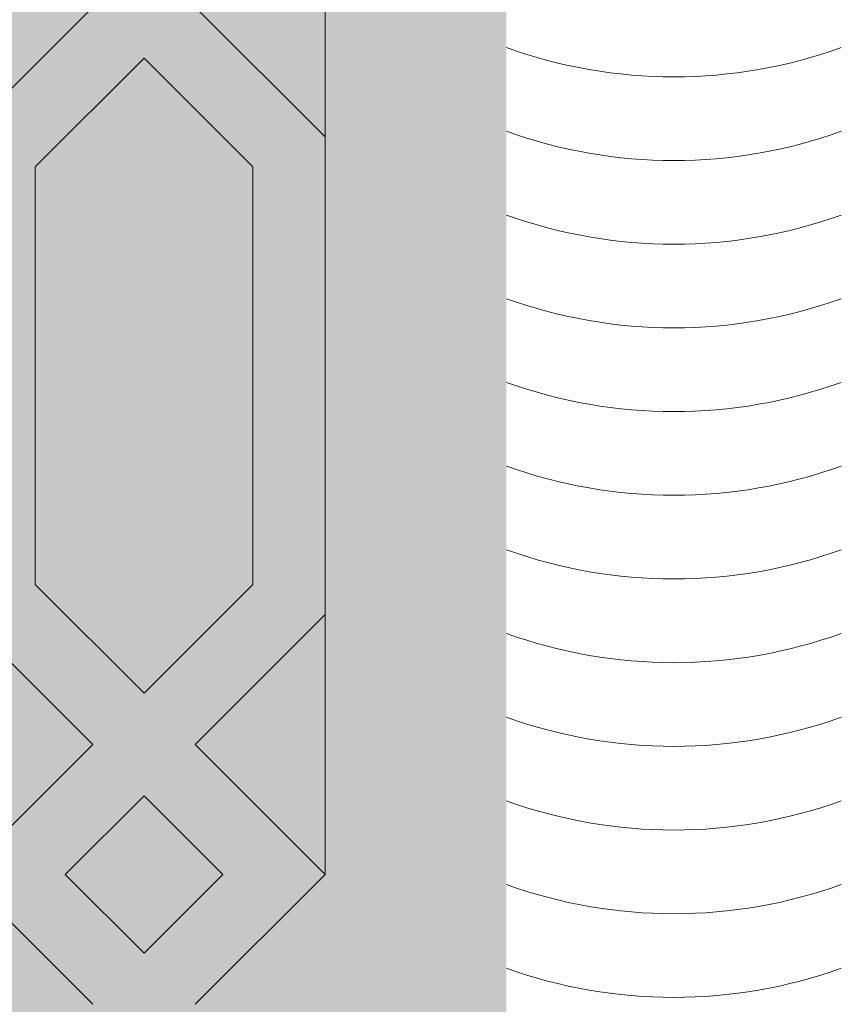
# Model space of a CAD drawing. Units: inches. Extents: x 844 to 2234, y 346 to 1084.
# Tile 37 of 93: x 1262.676 to 1265.567, y 695.763 to 699.229. Entities that reach past the tile are written whole.
import ezdxf

# ---------------------------------------------------------------- set-up
doc = ezdxf.new("R2010")
doc.units = ezdxf.units.IN
doc.header["$MEASUREMENT"] = 0
doc.layers.add('furniture', color=8, linetype='Continuous', lineweight=18)
doc.layers.add('RA-AP-01$0$INT', color=35, linetype='Continuous', lineweight=5)
doc.layers.add('RA-AP-01$0$FURN', color=3, linetype='Continuous')

# ---------------------------------------------------------------- blocks, each defined once
blk = doc.blocks.new('A$C18D01794')
at = {"layer": 'RA-AP-01$0$INT'}
h = blk.add_hatch(color=256, dxfattribs=at)
h.paths.add_polyline_path([(4.355206456958071, -6.156712009588037), (4.355206456958071, -8.056712009588038), (5.455206456958072, -8.056712009588038), (5.455206456958072, -6.156712009588037)])
h.paths.add_polyline_path([(4.405206456958072, -8.006712009588039), (4.405206456958072, -6.206712009588038), (5.405206456958072, -6.206712009588038), (5.405206456958072, -8.006712009588039)], flags=16)
h = blk.add_hatch(color=256, dxfattribs=at)
h.paths.add_polyline_path([(4.469348592586677, -7.07085414521094), (4.505206456958073, -7.03499628085108), (4.505206456958071, -7.106712009593861)])
h.paths.add_polyline_path([(4.455206456960671, -7.084996280832395), (4.476922185709333, -7.106712009588038), (4.433490728198045, -7.106712009588038)])
h.paths.add_polyline_path([(4.405206456958073, -7.034996280813718), (4.441064321339218, -7.070854145206393), (4.40520645695807, -7.106712009576003)])
h.paths.add_polyline_path([(4.425206456989053, -6.911460746921742), (4.455206456990736, -6.881460746929706), (4.485206456989055, -6.911460746937677), (4.48520645696979, -7.026712009590022), (4.455206456965227, -7.056712009584936), (4.425206456969784, -7.026712009579853)])
h.paths.add_polyline_path([(4.505206456958073, -6.831460746955388), (4.505206456958071, -6.903176475661116), (4.469348592616738, -6.867318611308251)])
h.paths.add_polyline_path([(4.425206456964688, -6.707925213036777), (4.455206456964794, -6.677925213027025), (4.485206456964689, -6.707925213017265), (4.485206456983951, -6.823176475683938), (4.455206456990736, -6.853176475686799), (4.425206456983956, -6.823176475689667)])
h.paths.add_polyline_path([(4.425206456974126, -6.504389679118949), (4.455206456959092, -6.474389679124341), (4.485206456974132, -6.504389679129721), (4.485206456993396, -6.619640941768059), (4.45520645699153, -6.649640941779566), (4.425206456993394, -6.619640941791077)])
h.paths.add_polyline_path([(4.46934859260189, -6.663783077416661), (4.505206456958071, -6.627925213048953), (4.505206456958073, -6.699640941761311)])
h.paths.add_polyline_path([(4.405206456958073, -6.627925213005104), (4.441064321354427, -6.663783077389926), (4.405206456958072, -6.699640941797813)])
h.paths.add_polyline_path([(4.405206456958072, -6.424389679139403), (4.441064321333084, -6.460247543502882), (4.405206456958072, -6.496105407889427)])
h.paths.add_polyline_path([(4.469348592580547, -6.460247543498336), (4.505206456958071, -6.424389679109282), (4.505206456958071, -6.496105407864332)])
h.paths.add_polyline_path([(4.425206456957888, -6.300854145208262), (4.45520645695415, -6.270854145221655), (4.485206456959507, -6.300854145217359), (4.48520645695824, -6.416105407863534), (4.455206456954537, -6.44610540787688), (4.425206456957888, -6.416105407889874)])
h.paths.add_polyline_path([(4.425206456957888, -6.226712009591025), (4.471064321332215, -6.226712009591025), (4.425206456957888, -6.272569873980103)])
h.paths.add_polyline_path([(4.499348592575121, -6.226712009591029), (4.636064321343707, -6.226712009591025), (4.666064321342317, -6.256712009589254), (4.636064321340932, -6.286712009591028), (4.499348592588945, -6.286712009591028), (4.469348592591685, -6.256712009584116)])
h.paths.add_polyline_path([(4.680206456964641, -6.270854145214393), (4.716064321337824, -6.306712009588038), (4.644348592591454, -6.306712009588038)])
h.paths.add_polyline_path([(4.644348592588108, -6.206712009588038), (4.716064321341167, -6.206712009588038), (4.680206456964637, -6.242569873964111)])
h.paths.add_polyline_path([(4.724348592586768, -6.226712009589824), (4.861064321340514, -6.226712009589824), (4.891064321340324, -6.256712009589255), (4.861064321340141, -6.286712009589827), (4.724348592587134, -6.286712009589821), (4.694348592586957, -6.256712009589254)])
h.paths.add_polyline_path([(4.905206456964143, -6.270854145212892), (4.941064321338827, -6.306712009588038), (4.869348592589457, -6.306712009588039)])
h.paths.add_polyline_path([(4.869348592586113, -6.206712009588038), (4.941064321342172, -6.206712009588038), (4.905206456964145, -6.242569873965612)])
h.paths.add_polyline_path([(4.949348592587774, -6.226712009589824), (5.086064321341521, -6.226712009589824), (5.116064321341329, -6.256712009589252), (5.08606432134115, -6.286712009589823), (4.949348592588145, -6.286712009589827), (4.919348592587961, -6.256712009589255)])
h.paths.add_polyline_path([(5.130206456963645, -6.270854145214393), (5.166064321336834, -6.306712009588038), (5.094348592590464, -6.306712009588038)])
h.paths.add_polyline_path([(5.094348592587119, -6.206712009588038), (5.166064321340178, -6.206712009588038), (5.130206456963651, -6.242569873964107)])
h.paths.add_polyline_path([(5.174348592584578, -6.226712009591027), (5.311064321353163, -6.226712009591027), (5.341064321336602, -6.256712009584116), (5.31106432133934, -6.286712009591028), (5.174348592587352, -6.286712009591028), (5.144348592585969, -6.256712009589254)])
h.paths.add_polyline_path([(5.325206456968778, -6.300854145217359), (5.355206456974136, -6.270854145221653), (5.385206456970396, -6.300854145208262), (5.385206456970396, -6.416105407889878), (5.355206456973747, -6.44610540787688), (5.325206456970044, -6.416105407863533)])
h.paths.add_polyline_path([(5.339348592596073, -6.226712009591029), (5.385206456970396, -6.226712009591025), (5.385206456970398, -6.272569873980105)])
h.paths.add_polyline_path([(5.325206456954155, -6.504389679129722), (5.355206456969194, -6.474389679124342), (5.38520645695416, -6.504389679118949), (5.385206456934896, -6.619640941791077), (5.355206456936758, -6.649640941779564), (5.325206456934888, -6.619640941768057)])
h.paths.add_polyline_path([(5.305206456958072, -6.424389679097139), (5.341064321347739, -6.460247543498338), (5.305206456958072, -6.496105407876472)])
h.paths.add_polyline_path([(5.369348592595204, -6.460247543502882), (5.40520645695807, -6.42438967915155), (5.405206456958072, -6.496105407877278)])
h.paths.add_polyline_path([(5.405206456958072, -6.627925213017245), (5.405206456958072, -6.69964094178567), (5.369348592573857, -6.663783077389926)])
h.paths.add_polyline_path([(5.305206456958072, -6.62792521303681), (5.341064321326393, -6.663783077416663), (5.305206456958072, -6.69964094177345)])
h.paths.add_polyline_path([(5.325206456963599, -6.707925213017267), (5.355206456963494, -6.677925213027021), (5.385206456963598, -6.707925213036775), (5.385206456944334, -6.823176475689665), (5.355206456937552, -6.853176475686797), (5.325206456944333, -6.823176475683936)])
h.paths.add_polyline_path([(5.305206456958072, -6.831460746943246), (5.341064321311551, -6.867318611308252), (5.305206456958072, -6.903176475673257)])
h.paths.add_polyline_path([(5.325206456939231, -6.911460746937672), (5.355206456937552, -6.881460746929707), (5.385206456939235, -6.911460746921742), (5.385206456958502, -7.026712009579853), (5.355206456963061, -7.056712009584934), (5.3252064569585, -7.026712009590026)])
h.paths.add_polyline_path([(5.404581768715993, -6.832085435167151, 0.001217816984214), (5.405206456958072, -6.832312009593747), (5.405206456958072, -6.90317647569123), (5.369348592563558, -6.867318611308251)])
h.paths.add_polyline_path([(5.36934859258907, -7.070854145206393), (5.40520645695807, -7.034996280825861), (5.405206456958072, -7.106712009563858)])
h.paths.add_polyline_path([(5.355206456967613, -7.084996280832394), (5.376922185730239, -7.106712009588038), (5.333490728218953, -7.106712009588036)])
h.paths.add_polyline_path([(5.30520645695807, -7.034996280838937), (5.341064321341609, -7.070854145210942), (5.305206456958074, -7.106712009606006)])
h = blk.add_hatch(color=256, dxfattribs=at)
h.paths.add_polyline_path([(4.505206456958071, -6.627925213048953), (4.46934859260189, -6.663783077416663), (4.505206456958071, -6.699640941761309), (4.505206456958071, -6.831460746955389), (4.469348592616735, -6.867318611308252), (4.505206456958071, -6.903176475661112), (4.505206456958071, -7.03499628085108), (4.469348592586679, -7.070854145210939), (4.505206456952245, -7.106712009588038), (4.476922185709333, -7.106712009588038), (4.455206456960671, -7.084996280832395), (4.433490728198047, -7.106712009588038), (4.405206456946033, -7.10671200958804), (4.441064321339216, -7.070854145206393), (4.40520645695807, -7.034996280813718), (4.405206456958072, -6.903176475703379), (4.441064321364728, -6.867318611308251), (4.40520645695807, -6.83146074691313), (4.40520645695807, -6.699640941797813), (4.441064321354429, -6.663783077389924), (4.405206456958072, -6.627925213005102), (4.405206456958072, -6.496105407889425), (4.441064321333084, -6.460247543502882), (4.405206456958072, -6.424389679139403), (4.405206456958072, -6.206712009588038), (4.644348592588106, -6.206712009588038), (4.680206456964639, -6.242569873964107), (4.716064321341165, -6.206712009588038), (4.869348592586113, -6.206712009588038), (4.905206456964143, -6.24256987396561), (4.941064321342174, -6.206712009588038), (5.094348592587118, -6.206712009588038), (5.130206456963649, -6.242569873964107), (5.166064321340178, -6.206712009588038), (5.405206456958072, -6.206712009588038), (5.405206456958072, -6.42438967915155), (5.369348592595202, -6.46024754350288), (5.40520645695807, -6.49610540787728), (5.40520645695807, -6.627925213017247), (5.369348592573859, -6.663783077389926), (5.40520645695807, -6.699640941785666), (5.40520645695807, -6.831460746925273), (5.36934859256356, -6.867318611308252), (5.405206456958072, -6.90317647569123), (5.405206456958072, -7.034996280825859), (5.369348592589068, -7.070854145206395), (5.405206456982249, -7.106712009588038), (5.376922185730244, -7.106712009588038), (5.355206456967613, -7.084996280832397), (5.333490728218955, -7.106712009588036), (5.305206456976043, -7.106712009588035), (5.341064321341609, -7.07085414521094), (5.305206456958072, -7.034996280838935), (5.305206456958072, -6.90317647567326), (5.34106432131155, -6.867318611308252), (5.305206456958072, -6.831460746943244), (5.30520645695807, -6.699640941773452), (5.341064321326395, -6.663783077416663), (5.305206456958072, -6.627925213036814), (5.305206456958072, -6.496105407876472), (5.341064321347738, -6.46024754349834), (5.305206456958072, -6.424389679097137), (5.30520645695807, -6.306712009588038), (5.166064321336834, -6.306712009588038), (5.130206456963647, -6.270854145214393), (5.094348592590464, -6.306712009588038), (4.941064321338827, -6.306712009588036), (4.905206456964145, -6.270854145212892), (4.869348592589459, -6.306712009588038), (4.716064321337822, -6.306712009588036), (4.680206456964641, -6.270854145214393), (4.644348592591453, -6.306712009588038), (4.505206456958071, -6.306712009588038), (4.505206456958071, -6.424389679109282), (4.469348592580545, -6.460247543498338), (4.505206456958071, -6.496105407864328)])
h.paths.add_polyline_path([(4.485206456974132, -6.504389679129722), (4.45520645695909, -6.474389679124341), (4.425206456974128, -6.504389679118945), (4.425206456993394, -6.619640941791079), (4.45520645699153, -6.649640941779566), (4.485206456993396, -6.619640941768059)], flags=16)
h.paths.add_polyline_path([(4.455206456954537, -6.44610540787688), (4.485206456958242, -6.416105407863534), (4.48520645695951, -6.30085414521736), (4.45520645695415, -6.270854145221653), (4.425206456957888, -6.300854145208264), (4.425206456957888, -6.41610540788988)], flags=16)
h.paths.add_polyline_path([(4.455206456964794, -6.677925213027025), (4.42520645696469, -6.707925213036777), (4.425206456983954, -6.82317647568967), (4.455206456990734, -6.853176475686797), (4.485206456983953, -6.823176475683936), (4.485206456964687, -6.707925213017265)], flags=16)
h.paths.add_polyline_path([(4.499348592588947, -6.286712009591028), (4.636064321340932, -6.286712009591028), (4.666064321342317, -6.256712009589254), (4.636064321343707, -6.226712009591027), (4.499348592575121, -6.226712009591029), (4.469348592591685, -6.256712009584118)], flags=16)
h.paths.add_polyline_path([(4.425206456957888, -6.272569873980103), (4.471064321332215, -6.226712009591025), (4.425206456957888, -6.226712009591025)], flags=16)
h.paths.add_polyline_path([(4.455206456990734, -6.881460746929709), (4.425206456989053, -6.91146074692174), (4.425206456969784, -7.026712009579853), (4.455206456965226, -7.056712009584932), (4.485206456969787, -7.026712009590026), (4.485206456989053, -6.911460746937672)], flags=16)
h.paths.add_polyline_path([(4.72434859258714, -6.286712009589821), (4.861064321340141, -6.286712009589829), (4.891064321340324, -6.256712009589254), (4.861064321340513, -6.226712009589823), (4.724348592586768, -6.226712009589823), (4.694348592586956, -6.256712009589254)], flags=16)
h.paths.add_polyline_path([(4.919348592587961, -6.256712009589254), (4.949348592588145, -6.286712009589827), (5.08606432134115, -6.286712009589823), (5.116064321341327, -6.256712009589254), (5.086064321341519, -6.226712009589824), (4.949348592587774, -6.226712009589824)], flags=16)
h.paths.add_polyline_path([(5.144348592585967, -6.256712009589254), (5.174348592587358, -6.286712009591028), (5.311064321339338, -6.286712009591028), (5.3410643213366, -6.256712009584118), (5.311064321353163, -6.226712009591029), (5.174348592584576, -6.226712009591027)], flags=16)
h.paths.add_polyline_path([(5.32520645693489, -6.619640941768055), (5.355206456936755, -6.649640941779566), (5.385206456934894, -6.619640941791079), (5.38520645695416, -6.504389679118949), (5.355206456969194, -6.474389679124341), (5.325206456954153, -6.504389679129724)], flags=16)
h.paths.add_polyline_path([(5.325206456970042, -6.416105407863534), (5.355206456973747, -6.44610540787688), (5.385206456970398, -6.416105407889876), (5.385206456970398, -6.30085414520826), (5.355206456974136, -6.270854145221653), (5.325206456968778, -6.30085414521736)], flags=16)
h.paths.add_polyline_path([(5.325206456963599, -6.707925213017265), (5.325206456944333, -6.823176475683936), (5.355206456937552, -6.853176475686797), (5.385206456944332, -6.823176475689667), (5.385206456963596, -6.707925213036773), (5.355206456963492, -6.677925213027027)], flags=16)
h.paths.add_polyline_path([(5.32520645693923, -6.911460746937674), (5.3252064569585, -7.026712009590026), (5.355206456963062, -7.056712009584934), (5.3852064569585, -7.026712009579853), (5.385206456939234, -6.911460746921738), (5.355206456937552, -6.881460746929707)], flags=16)
h.paths.add_polyline_path([(5.339348592596071, -6.226712009591029), (5.385206456970398, -6.272569873980103), (5.385206456970396, -6.226712009591027)], flags=16)
h = blk.add_hatch(color=256, dxfattribs=at)
h.paths.add_polyline_path([(4.505206456958071, -7.585498806127123), (4.46934859260189, -7.549640941759413), (4.505206456958071, -7.513783077414768), (4.505206456958071, -7.381963272220687), (4.469348592616735, -7.346105407867824), (4.505206456958071, -7.310247543514964), (4.505206456958071, -7.178427738324996), (4.469348592586679, -7.142569873965138), (4.505206456952245, -7.106712009588038), (4.476922185709333, -7.106712009588038), (4.455206456960671, -7.128427738343681), (4.433490728198047, -7.106712009588038), (4.405206456946033, -7.106712009588036), (4.441064321339216, -7.142569873969684), (4.40520645695807, -7.178427738362358), (4.405206456958072, -7.310247543472698), (4.441064321364728, -7.346105407867826), (4.40520645695807, -7.381963272262947), (4.40520645695807, -7.513783077378263), (4.441064321354429, -7.549640941786153), (4.405206456958072, -7.585498806170974), (4.405206456958072, -7.717318611286652), (4.441064321333084, -7.753176475673194), (4.405206456958072, -7.789034340036673), (4.405206456958072, -8.006712009588039), (4.644348592588106, -8.006712009588039), (4.680206456964639, -7.970854145211967), (4.716064321341165, -8.006712009588039), (4.869348592586113, -8.006712009588039), (4.905206456964143, -7.970854145210465), (4.941064321342174, -8.006712009588039), (5.094348592587118, -8.006712009588037), (5.130206456963649, -7.970854145211967), (5.166064321340178, -8.006712009588039), (5.405206456958072, -8.006712009588039), (5.405206456958072, -7.789034340024526), (5.369348592595202, -7.753176475673196), (5.40520645695807, -7.717318611298797), (5.40520645695807, -7.585498806158829), (5.369348592573859, -7.549640941786151), (5.40520645695807, -7.51378307739041), (5.40520645695807, -7.381963272250803), (5.36934859256356, -7.346105407867824), (5.405206456958072, -7.310247543484846), (5.405206456958072, -7.178427738350217), (5.369348592589068, -7.142569873969682), (5.405206456982249, -7.106712009588038), (5.376922185730244, -7.106712009588038), (5.355206456967613, -7.128427738343679), (5.333490728218955, -7.10671200958804), (5.305206456976043, -7.106712009588042), (5.341064321341609, -7.142569873965136), (5.305206456958072, -7.178427738337141), (5.305206456958072, -7.310247543502816), (5.34106432131155, -7.346105407867824), (5.305206456958072, -7.381963272232832), (5.30520645695807, -7.513783077402624), (5.341064321326395, -7.549640941759413), (5.305206456958072, -7.585498806139263), (5.305206456958072, -7.717318611299605), (5.341064321347738, -7.753176475677737), (5.305206456958072, -7.78903434007894), (5.30520645695807, -7.906712009588039), (5.166064321336834, -7.906712009588039), (5.130206456963647, -7.942569873961684), (5.094348592590464, -7.906712009588039), (4.941064321338827, -7.906712009588041), (4.905206456964145, -7.942569873963183), (4.869348592589459, -7.906712009588039), (4.716064321337822, -7.906712009588041), (4.680206456964641, -7.942569873961684), (4.644348592591453, -7.906712009588039), (4.505206456958071, -7.906712009588039), (4.505206456958071, -7.789034340066795), (4.469348592580545, -7.753176475677738), (4.505206456958071, -7.717318611311748)])
h.paths.add_polyline_path([(4.485206456974132, -7.709034340046354), (4.45520645695909, -7.739034340051736), (4.425206456974128, -7.709034340057131), (4.425206456993394, -7.593783077384998), (4.45520645699153, -7.563783077396511), (4.485206456993396, -7.593783077408017)], flags=16)
h.paths.add_polyline_path([(4.455206456954537, -7.767318611299197), (4.485206456958242, -7.797318611312542), (4.48520645695951, -7.912569873958716), (4.45520645695415, -7.942569873954422), (4.425206456957888, -7.912569873967813), (4.425206456957888, -7.797318611286197)], flags=16)
h.paths.add_polyline_path([(4.455206456964794, -7.535498806149051), (4.42520645696469, -7.5054988061393), (4.425206456983954, -7.390247543486406), (4.455206456990734, -7.360247543489279), (4.485206456983953, -7.39024754349214), (4.485206456964687, -7.505498806158811)], flags=16)
h.paths.add_polyline_path([(4.499348592588947, -7.926712009585049), (4.636064321340932, -7.926712009585049), (4.666064321342317, -7.956712009586821), (4.636064321343707, -7.986712009585048), (4.499348592575121, -7.986712009585048), (4.469348592591685, -7.956712009591957)], flags=16)
h.paths.add_polyline_path([(4.425206456957888, -7.940854145195974), (4.471064321332215, -7.986712009585049), (4.425206456957888, -7.986712009585049)], flags=16)
h.paths.add_polyline_path([(4.455206456990734, -7.331963272246367), (4.425206456989053, -7.301963272254337), (4.425206456969784, -7.186712009596224), (4.455206456965226, -7.156712009591144), (4.485206456969787, -7.186712009586051), (4.485206456989053, -7.301963272238404)], flags=16)
h.paths.add_polyline_path([(4.72434859258714, -7.926712009586255), (4.861064321340141, -7.926712009586248), (4.891064321340324, -7.956712009586823), (4.861064321340513, -7.986712009586252), (4.724348592586768, -7.986712009586252), (4.694348592586956, -7.956712009586821)], flags=16)
h.paths.add_polyline_path([(4.919348592587961, -7.956712009586821), (4.949348592588145, -7.92671200958625), (5.08606432134115, -7.926712009586253), (5.116064321341327, -7.956712009586823), (5.086064321341519, -7.986712009586252), (4.949348592587774, -7.986712009586252)], flags=16)
h.paths.add_polyline_path([(5.144348592585967, -7.956712009586823), (5.174348592587358, -7.926712009585049), (5.311064321339338, -7.926712009585049), (5.3410643213366, -7.956712009591957), (5.311064321353163, -7.986712009585048), (5.174348592584576, -7.986712009585048)], flags=16)
h.paths.add_polyline_path([(5.32520645693489, -7.593783077408021), (5.355206456936755, -7.563783077396511), (5.385206456934894, -7.593783077384998), (5.38520645695416, -7.709034340057128), (5.355206456969194, -7.739034340051736), (5.325206456954153, -7.709034340046352)], flags=16)
h.paths.add_polyline_path([(5.325206456970042, -7.797318611312542), (5.355206456973747, -7.767318611299197), (5.385206456970398, -7.7973186112862), (5.385206456970398, -7.912569873967816), (5.355206456974136, -7.942569873954422), (5.325206456968778, -7.912569873958716)], flags=16)
h.paths.add_polyline_path([(5.325206456963599, -7.505498806158811), (5.325206456944333, -7.39024754349214), (5.355206456937552, -7.360247543489279), (5.385206456944332, -7.39024754348641), (5.385206456963596, -7.505498806139303), (5.355206456963492, -7.53549880614905)], flags=16)
h.paths.add_polyline_path([(5.32520645693923, -7.301963272238403), (5.3252064569585, -7.186712009586051), (5.355206456963062, -7.156712009591142), (5.3852064569585, -7.186712009596224), (5.385206456939234, -7.301963272254338), (5.355206456937552, -7.331963272246369)], flags=16)
h.paths.add_polyline_path([(5.339348592596071, -7.986712009585048), (5.385206456970398, -7.940854145195972), (5.385206456970396, -7.986712009585048)], flags=16)
h = blk.add_hatch(color=256, dxfattribs=at)
h.paths.add_polyline_path([(4.469348592586677, -7.142569873965136), (4.505206456958073, -7.178427738324996), (4.505206456958071, -7.106712009582215)])
h.paths.add_polyline_path([(4.455206456960671, -7.128427738343681), (4.476922185709333, -7.106712009588038), (4.433490728198045, -7.106712009588038)])
h.paths.add_polyline_path([(4.405206456958073, -7.178427738362358), (4.441064321339218, -7.142569873969684), (4.40520645695807, -7.106712009600073)])
h.paths.add_polyline_path([(4.425206456989053, -7.301963272254335), (4.455206456990736, -7.331963272246371), (4.485206456989055, -7.301963272238399), (4.48520645696979, -7.186712009586054), (4.455206456965227, -7.15671200959114), (4.425206456969784, -7.186712009596224)])
h.paths.add_polyline_path([(4.505206456958073, -7.381963272220689), (4.505206456958071, -7.310247543514961), (4.469348592616738, -7.346105407867826)])
h.paths.add_polyline_path([(4.425206456964688, -7.5054988061393), (4.455206456964794, -7.535498806149051), (4.485206456964689, -7.505498806158811), (4.485206456983951, -7.390247543492138), (4.455206456990736, -7.360247543489277), (4.425206456983956, -7.39024754348641)])
h.paths.add_polyline_path([(4.425206456974126, -7.709034340057128), (4.455206456959092, -7.739034340051736), (4.485206456974132, -7.709034340046356), (4.485206456993396, -7.593783077408017), (4.45520645699153, -7.563783077396511), (4.425206456993394, -7.593783077384999)])
h.paths.add_polyline_path([(4.46934859260189, -7.549640941759415), (4.505206456958071, -7.585498806127123), (4.505206456958073, -7.513783077414766)])
h.paths.add_polyline_path([(4.405206456958073, -7.585498806170972), (4.441064321354427, -7.549640941786151), (4.405206456958072, -7.513783077378263)])
h.paths.add_polyline_path([(4.405206456958072, -7.789034340036673), (4.441064321333084, -7.753176475673194), (4.405206456958072, -7.71731861128665)])
h.paths.add_polyline_path([(4.469348592580547, -7.75317647567774), (4.505206456958071, -7.789034340066795), (4.505206456958071, -7.717318611311744)])
h.paths.add_polyline_path([(4.425206456957888, -7.912569873967814), (4.45520645695415, -7.942569873954422), (4.485206456959507, -7.912569873958718), (4.48520645695824, -7.797318611312542), (4.455206456954537, -7.767318611299197), (4.425206456957888, -7.797318611286202)])
h.paths.add_polyline_path([(4.425206456957888, -7.986712009585049), (4.471064321332215, -7.986712009585049), (4.425206456957888, -7.940854145195972)])
h.paths.add_polyline_path([(4.499348592575121, -7.986712009585048), (4.636064321343707, -7.986712009585049), (4.666064321342317, -7.956712009586823), (4.636064321340932, -7.926712009585049), (4.499348592588945, -7.926712009585049), (4.469348592591685, -7.95671200959196)])
h.paths.add_polyline_path([(4.680206456964641, -7.942569873961684), (4.716064321337824, -7.906712009588039), (4.644348592591454, -7.906712009588039)])
h.paths.add_polyline_path([(4.644348592588108, -8.006712009588039), (4.716064321341167, -8.006712009588039), (4.680206456964637, -7.970854145211964)])
h.paths.add_polyline_path([(4.724348592586768, -7.98671200958625), (4.861064321340514, -7.986712009586252), (4.891064321340324, -7.956712009586819), (4.861064321340141, -7.92671200958625), (4.724348592587134, -7.926712009586255), (4.694348592586957, -7.956712009586821)])
h.paths.add_polyline_path([(4.905206456964143, -7.942569873963183), (4.941064321338827, -7.906712009588039), (4.869348592589457, -7.906712009588037)])
h.paths.add_polyline_path([(4.869348592586113, -8.006712009588039), (4.941064321342172, -8.006712009588037), (4.905206456964145, -7.970854145210463)])
h.paths.add_polyline_path([(4.949348592587774, -7.986712009586252), (5.086064321341521, -7.986712009586252), (5.116064321341329, -7.956712009586823), (5.08606432134115, -7.926712009586253), (4.949348592588145, -7.92671200958625), (4.919348592587961, -7.956712009586819)])
h.paths.add_polyline_path([(5.130206456963645, -7.942569873961684), (5.166064321336834, -7.906712009588039), (5.094348592590464, -7.906712009588039)])
h.paths.add_polyline_path([(5.094348592587119, -8.006712009588039), (5.166064321340178, -8.006712009588039), (5.130206456963651, -7.970854145211967)])
h.paths.add_polyline_path([(5.174348592584578, -7.986712009585048), (5.311064321353163, -7.986712009585048), (5.341064321336602, -7.956712009591958), (5.31106432133934, -7.926712009585049), (5.174348592587352, -7.926712009585049), (5.144348592585969, -7.956712009586823)])
h.paths.add_polyline_path([(5.325206456968778, -7.912569873958718), (5.355206456974136, -7.942569873954422), (5.385206456970396, -7.912569873967814), (5.385206456970396, -7.797318611286199), (5.355206456973747, -7.767318611299197), (5.325206456970044, -7.797318611312544)])
h.paths.add_polyline_path([(5.339348592596073, -7.986712009585048), (5.385206456970396, -7.986712009585049), (5.385206456970398, -7.94085414519597)])
h.paths.add_polyline_path([(5.325206456954155, -7.709034340046354), (5.355206456969194, -7.739034340051734), (5.38520645695416, -7.709034340057128), (5.385206456934896, -7.593783077384999), (5.355206456936758, -7.563783077396513), (5.325206456934888, -7.593783077408019)])
h.paths.add_polyline_path([(5.305206456958072, -7.789034340078938), (5.341064321347739, -7.753176475677738), (5.305206456958072, -7.717318611299605)])
h.paths.add_polyline_path([(5.369348592595204, -7.753176475673194), (5.40520645695807, -7.789034340024526), (5.405206456958072, -7.717318611298798)])
h.paths.add_polyline_path([(5.405206456958072, -7.585498806158831), (5.405206456958072, -7.513783077390407), (5.369348592573857, -7.549640941786151)])
h.paths.add_polyline_path([(5.305206456958072, -7.585498806139266), (5.341064321326393, -7.549640941759413), (5.305206456958072, -7.513783077402626)])
h.paths.add_polyline_path([(5.325206456963599, -7.50549880615881), (5.355206456963494, -7.535498806149055), (5.385206456963598, -7.505498806139302), (5.385206456944334, -7.390247543486411), (5.355206456937552, -7.360247543489279), (5.325206456944333, -7.39024754349214)])
h.paths.add_polyline_path([(5.305206456958072, -7.38196327223283), (5.341064321311551, -7.346105407867824), (5.305206456958072, -7.31024754350282)])
h.paths.add_polyline_path([(5.325206456939231, -7.301963272238404), (5.355206456937552, -7.331963272246369), (5.385206456939235, -7.301963272254335), (5.385206456958502, -7.186712009596224), (5.355206456963061, -7.156712009591142), (5.3252064569585, -7.186712009586051)])
h.paths.add_polyline_path([(5.404581768715993, -7.381338584008926, -0.001217816984214), (5.405206456958072, -7.381112009582329), (5.405206456958072, -7.310247543484846), (5.369348592563558, -7.346105407867826)])
h.paths.add_polyline_path([(5.36934859258907, -7.142569873969684), (5.40520645695807, -7.178427738350215), (5.405206456958072, -7.106712009612218)])
h.paths.add_polyline_path([(5.355206456967613, -7.128427738343683), (5.376922185730239, -7.106712009588038), (5.333490728218953, -7.10671200958804)])
h.paths.add_polyline_path([(5.30520645695807, -7.178427738337139), (5.341064321341609, -7.142569873965134), (5.305206456958074, -7.10671200957007)])
blk.add_hatch(color=256, dxfattribs=at).paths.add_polyline_path([(4.405206456958072, -7.381963272262946), (4.441064321364729, -7.346105407867824), (4.405206456958072, -7.310247543472702)])
for p, q in [((4.441064321339218, -7.070854145206393), (4.405206456956286, -7.106712009577787)), ((4.469348592586677, -7.07085414521094), (4.505206456958071, -7.106712009593865)), ((4.455206456960673, -7.084996280832395), (4.433490728204252, -7.106712009581832)), ((4.455206456960673, -7.084996280832395), (4.476922185709333, -7.106712009588038)), ((4.441064321339218, -7.142569873969684), (4.405206456956286, -7.10671200959829)), ((4.455206456960673, -7.128427738343681), (4.433490728204252, -7.106712009594245)), ((4.455206456960673, -7.128427738343681), (4.476922185709333, -7.106712009588038)), ((4.469348592586677, -7.142569873965136), (4.505206456958071, -7.106712009582212)), ((4.405206456969147, -7.178427738351285), (4.441064321339218, -7.142569873969684)), ((4.505206456969147, -7.178427738336072), (4.469348592586681, -7.14256987396514)), ((4.425206456970426, -7.186712009595584), (4.455206456965226, -7.156712009591142)), ((4.485206456970428, -7.186712009586692), (4.455206456965226, -7.156712009591142)), ((4.425206456989053, -7.301963272254337), (4.425206456969786, -7.186712009596725)), ((4.485206456989055, -7.301963272238403), (4.485206456969787, -7.186712009586692)), ((4.425206456989053, -7.301963272254337), (4.455206456990734, -7.331963272246369)), ((4.485206456989055, -7.301963272238403), (4.455206456990734, -7.331963272246369)), ((4.405206456987673, -7.310247543502303), (4.441064321369275, -7.346105407872371)), ((4.505206456987672, -7.31024754348536), (4.469348592616737, -7.346105407867824))]:
    blk.add_line(p, q, dxfattribs=at)
blk.add_lwpolyline([(5.405206456958072, -8.006712009588039), (4.405206456958072, -8.006712009588039), (4.405206456958072, -7.106712009588038)], dxfattribs=at)
for centre in [(4.30900645695254, -7.20916445828451), (4.30900645695254, -7.232264458283259), (4.309006456955269, -7.255364458282008), (4.309006456955269, -7.278464458280756), (4.309006456953677, -7.301564458285417), (4.309006456954814, -7.324664458284166), (4.309006456954814, -7.347764458279732), (4.309006456953222, -7.37086445828462), (4.309006456955951, -7.393964458283369), (4.309006456955951, -7.417064458282117), (4.309006456954359, -7.440164458286778), (4.309006456955496, -7.463264458285527)]:
    blk.add_arc(centre, 0.136414042854523, 70.20384312815696, 109.7961568705686, dxfattribs=at)
blk = doc.blocks.new('A$C5D2F253E')
at = {"layer": 'RA-AP-01$0$FURN', "xscale": -0.7999999999883585, "yscale": 0.7999999999883585, "zscale": 0.8, "rotation": 90}
blk.add_blockref('A$C18D01794', (-5.687757199772477, 4.75791982714071), dxfattribs=at)

msp = doc.modelspace()

# ---------------------------------------------------------------- block references
at = {"layer": 'furniture', "xscale": -15.94108302203742, "yscale": 15.94108302203742, "zscale": 15.94108302203742, "rotation": 270}
msp.add_blockref('A$C5D2F253E', (1244.08405109492, 696.2584716700112), dxfattribs=at)

doc.saveas('drawing.dxf')
